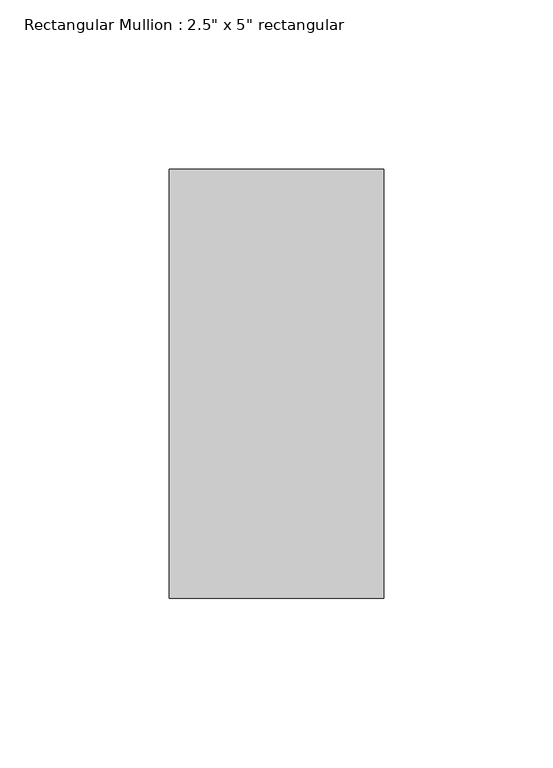
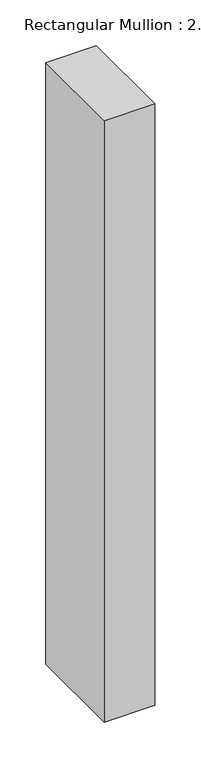
"""IFC4 building model written with IfcOpenShell, lengths in millimetres: member geometry."""

from ifc_helpers import new_model, si_unit, frame, origin, place, context, project, spatial, polyline, outline, extrude, source, transform, mapped, element, save


def member_d36207d9(model_context):
    return source(origin(), model_context, "Body", "SweptSolid", [
        extrude(outline(polyline([(0.0, 63.5), (0.0, -63.5), (-63.5, -63.5), (-63.5, 63.5), (0.0, 63.5)])), frame((0.0, 0.0, -800.1), z_axis=(0.0, 0.0, 1.0), x_axis=(1.0, 0.0, 0.0)), (0.0, 0.0, 1.0), 800.1),
    ])


if __name__ == "__main__":
    model = new_model("IFC4")
    model_context = context("Model", 3, world=origin())
    ifc_project = project(units=[si_unit("LENGTHUNIT", "METRE", prefix="MILLI")], contexts=[model_context])
    site = spatial("IfcSite", under=ifc_project)
    building = spatial("IfcBuilding", under=site)
    placement = place(None, origin())
    member_shape = member_d36207d9(model_context)
    element("IfcMember", 1, ObjectType="Rectangular Mullion : 2.5\" x 5\" rectangular", at=placement, inside=building, context=model_context, shape_type="MappedRepresentation", body=[
        mapped(member_shape, transform((0.0, 0.0, 0.0), x_axis=(1.0, 0.0, 0.0), y_axis=(0.0, 1.0, 0.0), z_axis=(0.0, 0.0, 1.0))),
    ])
    save(model, "model.ifc")

# Revit data of these elements
# Type "Rectangular Mullion : 2.5\" x 5\" rectangular"
#   built-in parameter 1007304 = 0.416667 (stored number, unit not read)
#   built-in parameter 1007301 = 0.104167 (stored number, unit not read)
#   built-in parameter 1007300 = 0.104167 (stored number, unit not read)
# Element 1 (IfcMember, "Rectangular Mullion : 2.5\" x 5\" rectangular")
#   Materials on its faces: "Aluminum"
# Materials
#   "Aluminum": class "Metal", colour RGB 247 247 247, transparency 0, Description = "Aluminum 6061", Cost = 0
